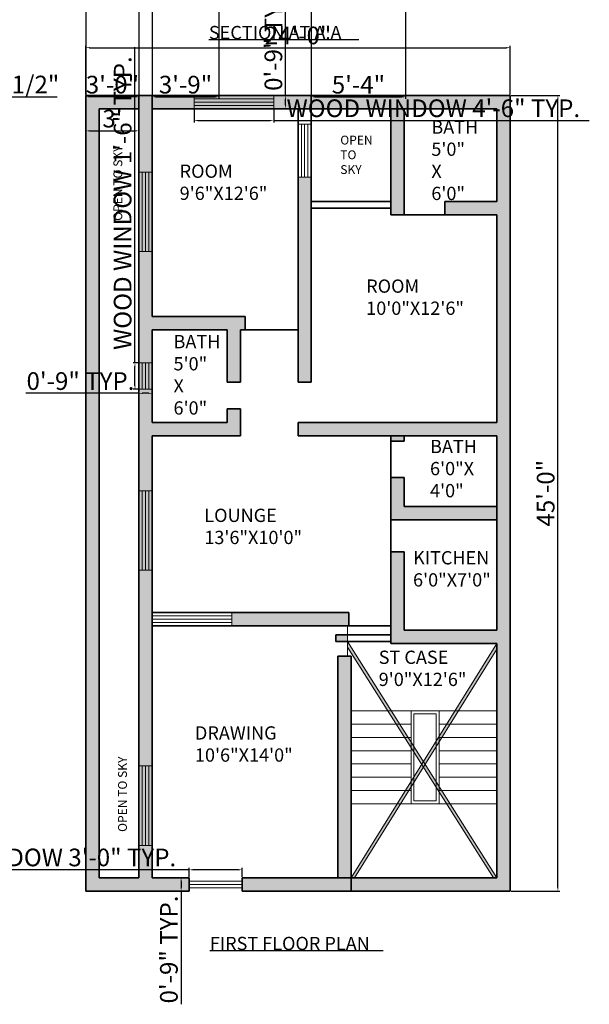
# Model space of a CAD drawing. Units: inches. Extents: x 2693 to 3501, y 1190 to 2292.
# Tile 2 of 4: x 3068 to 3455, y 1190 to 1858. Entities that reach past the tile are written whole.
import ezdxf

# ---------------------------------------------------------------- set-up
doc = ezdxf.new("R2010")
doc.units = ezdxf.units.IN
for name, color, linetype, lineweight in [('A-ANNO-DIMS', 2, 'Continuous', 18), ('A-ANNO-TEXT', 7, 'Continuous', 25), ('A-AREA-IDEN', 7, 'Continuous', 18), ('A-FLOR-STRS', 7, 'Continuous', 18), ('A-FLOR-STRS-PATT', 252, 'Continuous', 13), ('A-GLAZ', 4, 'Continuous', 18), ('A-WALL', 7, 'Continuous', 35), ('A-WALL-PATT', 252, 'Continuous', 13)]:
    doc.layers.add(name, color=color, linetype=linetype, lineweight=lineweight)
doc.styles.get("Standard").update_dxf_attribs({"font": 'arial.ttf'})
doc.dimstyles.new('ISO-25', dxfattribs={"dimtxt": 12, "dimasz": 2.5, "dimexe": 1.25, "dimexo": 0.625, "dimtad": 1, "dimdec": 1, "dimlunit": 3, "dimtxsty": 'Standard', "dimcen": 2.5, "dimadec": 0, "dimazin": 0, "dimtfac": 1, "dimtdec": 1, "dimtmove": 0, "dimatfit": 3, "dimfxl": 1, "dimarcsym": 0})

# ---------------------------------------------------------------- blocks, each defined once
blk = doc.blocks.new('Window - Wood Frame 36 in. Wide plan')
for p, q in [((0, 6), (0, 0)), ((0, 4.5), (36, 4.5)), ((36, 6), (36, 0)), ((0, 3), (36, 3)), ((0, 1.5), (36, 1.5))]:
    blk.add_line(p, q)
blk = doc.blocks.new('*D5')
at = {"layer": 'A-ANNO-DIMS', "color": 0, "lineweight": -2, "transparency": 16777216}
for p, q in [((3113.27, 1805.91), (3113.27, 1781.23)), ((3149.27, 1796.91), (3149.27, 1781.23)), ((3115.77, 1782.48), (3146.77, 1782.48))]:
    blk.add_line(p, q, dxfattribs=at)
at = {"layer": 'A-ANNO-DIMS', "color": 0, "transparency": 16777216}
for points in [[(3115.77, 1782.9), (3115.77, 1782.06), (3113.27, 1782.48)], [(3146.77, 1782.9), (3146.77, 1782.06), (3149.27, 1782.48)]]:
    blk.add_solid(points, dxfattribs=at)
at = {"layer": 'Defpoints', "color": 0, "transparency": 16777216}
for p in [(3113.27, 1806.53), (3149.27, 1797.53), (3149.27, 1782.48)]:
    blk.add_point(p, dxfattribs=at)
at = {"layer": 'A-ANNO-DIMS', "color": 0, "transparency": 16777216, "insert": (3131.27, 1789.23), "char_height": 12, "attachment_point": 5}
blk.add_mtext("3'", dxfattribs=at)
blk = doc.blocks.new('*D9')
at = {"layer": 'A-ANNO-DIMS', "color": 0, "lineweight": -2, "transparency": 16777216}
for p, q in [((3186.75, 1796.91), (3186.75, 1788.18)), ((3240.75, 1796.91), (3240.75, 1788.18)), ((3189.25, 1789.43), (3238.25, 1789.43)), ((3240.75, 1789.43), (3455.01, 1789.43))]:
    blk.add_line(p, q, dxfattribs=at)
at = {"layer": 'A-ANNO-DIMS', "color": 0, "transparency": 16777216}
for points in [[(3189.25, 1789.85), (3189.25, 1789.02), (3186.75, 1789.43)], [(3238.25, 1789.85), (3238.25, 1789.02), (3240.75, 1789.43)]]:
    blk.add_solid(points, dxfattribs=at)
at = {"layer": 'Defpoints', "color": 0, "transparency": 16777216}
for p in [(3186.75, 1797.53), (3240.75, 1797.53), (3240.75, 1789.43)]:
    blk.add_point(p, dxfattribs=at)
at = {"layer": 'A-ANNO-DIMS', "color": 0, "transparency": 16777216, "insert": (3349.13, 1796.27), "char_height": 12, "attachment_point": 5}
blk.add_mtext('WOOD WINDOW 4\'-6" TYP.', dxfattribs=at)
blk = doc.blocks.new('*D10')
at = {"layer": 'A-ANNO-DIMS', "color": 0, "lineweight": -2, "transparency": 16777216}
for p, q in [((3248.85, 1806.53), (3248.85, 1883.43)), ((3241.37, 1806.53), (3250.1, 1806.53)), ((3248.85, 1800.03), (3248.85, 1804.03)), ((3241.37, 1797.53), (3250.1, 1797.53))]:
    blk.add_line(p, q, dxfattribs=at)
at = {"layer": 'A-ANNO-DIMS', "color": 0, "transparency": 16777216}
for points in [[(3248.43, 1804.03), (3249.26, 1804.03), (3248.85, 1806.53)], [(3248.43, 1800.03), (3249.26, 1800.03), (3248.85, 1797.53)]]:
    blk.add_solid(points, dxfattribs=at)
at = {"layer": 'Defpoints', "color": 0, "transparency": 16777216}
for p in [(3240.75, 1806.53), (3248.85, 1806.53), (3240.75, 1797.53)]:
    blk.add_point(p, dxfattribs=at)
at = {"layer": 'A-ANNO-DIMS', "color": 0, "transparency": 16777216, "insert": (3242.09, 1846.23), "char_height": 12, "attachment_point": 5, "rotation": 90}
blk.add_mtext('0\'-9" TYP.', dxfattribs=at)
blk = doc.blocks.new('*D11')
at = {"layer": 'A-ANNO-DIMS', "color": 0, "lineweight": -2, "transparency": 16777216}
for p, q in [((3183.29, 1280.93), (2969.02, 1280.93)), ((3183.29, 1276.16), (3183.29, 1282.18)), ((3216.79, 1280.93), (3185.79, 1280.93)), ((3219.29, 1276.16), (3219.29, 1282.18))]:
    blk.add_line(p, q, dxfattribs=at)
at = {"layer": 'A-ANNO-DIMS', "color": 0, "transparency": 16777216}
for points in [[(3185.79, 1281.35), (3185.79, 1280.52), (3183.29, 1280.93)], [(3216.79, 1281.35), (3216.79, 1280.52), (3219.29, 1280.93)]]:
    blk.add_solid(points, dxfattribs=at)
at = {"layer": 'Defpoints', "color": 0, "transparency": 16777216}
for p in [(3183.29, 1280.93), (3183.29, 1275.53), (3219.29, 1275.53)]:
    blk.add_point(p, dxfattribs=at)
at = {"layer": 'A-ANNO-DIMS', "color": 0, "transparency": 16777216, "insert": (3074.91, 1287.77), "char_height": 12, "attachment_point": 5}
blk.add_mtext('WOOD WINDOW 3\'-0" TYP.', dxfattribs=at)
blk = doc.blocks.new('*D12')
at = {"layer": 'A-ANNO-DIMS', "color": 0, "lineweight": -2, "transparency": 16777216}
for p, q in [((3182.66, 1275.53), (3176.64, 1275.53)), ((3177.89, 1273.03), (3177.89, 1269.03)), ((3182.66, 1266.53), (3176.64, 1266.53)), ((3177.89, 1266.53), (3177.89, 1189.64))]:
    blk.add_line(p, q, dxfattribs=at)
at = {"layer": 'A-ANNO-DIMS', "color": 0, "transparency": 16777216}
for points in [[(3177.47, 1273.03), (3178.31, 1273.03), (3177.89, 1275.53)], [(3177.47, 1269.03), (3178.31, 1269.03), (3177.89, 1266.53)]]:
    blk.add_solid(points, dxfattribs=at)
at = {"layer": 'Defpoints', "color": 0, "transparency": 16777216}
for p in [(3183.29, 1275.53), (3177.89, 1266.53), (3183.29, 1266.53)]:
    blk.add_point(p, dxfattribs=at)
at = {"layer": 'A-ANNO-DIMS', "color": 0, "transparency": 16777216, "insert": (3171.14, 1226.84), "char_height": 12, "attachment_point": 5, "rotation": 90}
blk.add_mtext('0\'-9" TYP.', dxfattribs=at)
blk = doc.blocks.new('*D13')
at = {"layer": 'A-ANNO-DIMS', "color": 0, "lineweight": -2, "transparency": 16777216}
for p, q in [((3146.57, 1625.05), (3146.57, 1839.31)), ((3148.65, 1625.05), (3145.32, 1625.05)), ((3146.57, 1609.55), (3146.57, 1622.55)), ((3148.65, 1607.05), (3145.32, 1607.05))]:
    blk.add_line(p, q, dxfattribs=at)
at = {"layer": 'A-ANNO-DIMS', "color": 0, "transparency": 16777216}
for points in [[(3146.16, 1622.55), (3146.99, 1622.55), (3146.57, 1625.05)], [(3146.16, 1609.55), (3146.99, 1609.55), (3146.57, 1607.05)]]:
    blk.add_solid(points, dxfattribs=at)
at = {"layer": 'Defpoints', "color": 0, "transparency": 16777216}
for p in [(3146.57, 1625.05), (3149.27, 1625.05), (3149.27, 1607.05)]:
    blk.add_point(p, dxfattribs=at)
at = {"layer": 'A-ANNO-DIMS', "color": 0, "transparency": 16777216, "insert": (3139.74, 1733.43), "char_height": 12, "attachment_point": 5, "rotation": 90}
blk.add_mtext('WOOD WINDOW 1\'-6" TYP.', dxfattribs=at)
blk = doc.blocks.new('*D14')
at = {"layer": 'A-ANNO-DIMS', "color": 0, "lineweight": -2, "transparency": 16777216}
for p, q in [((3149.27, 1604.35), (3072.38, 1604.35)), ((3149.27, 1606.42), (3149.27, 1603.1)), ((3155.77, 1604.35), (3151.77, 1604.35)), ((3158.27, 1606.42), (3158.27, 1603.1))]:
    blk.add_line(p, q, dxfattribs=at)
at = {"layer": 'A-ANNO-DIMS', "color": 0, "transparency": 16777216}
for points in [[(3151.77, 1604.76), (3151.77, 1603.93), (3149.27, 1604.35)], [(3155.77, 1604.76), (3155.77, 1603.93), (3158.27, 1604.35)]]:
    blk.add_solid(points, dxfattribs=at)
at = {"layer": 'Defpoints', "color": 0, "transparency": 16777216}
for p in [(3149.27, 1607.05), (3149.27, 1604.35), (3158.27, 1607.05)]:
    blk.add_point(p, dxfattribs=at)
at = {"layer": 'A-ANNO-DIMS', "color": 0, "transparency": 16777216, "insert": (3109.57, 1611.1), "char_height": 12, "attachment_point": 5}
blk.add_mtext('0\'-9" TYP.', dxfattribs=at)
blk = doc.blocks.new('*D30')
at = {"layer": 'A-ANNO-DIMS', "color": 0, "lineweight": -2, "transparency": 16777216}
for p, q in [((3113.27, 1807.16), (3113.27, 1840.18)), ((3115.77, 1838.93), (3398.77, 1838.93)), ((3401.27, 1807.16), (3401.27, 1840.18))]:
    blk.add_line(p, q, dxfattribs=at)
at = {"layer": 'A-ANNO-DIMS', "color": 0, "transparency": 16777216}
for points in [[(3115.77, 1839.35), (3115.77, 1838.52), (3113.27, 1838.93)], [(3398.77, 1839.35), (3398.77, 1838.52), (3401.27, 1838.93)]]:
    blk.add_solid(points, dxfattribs=at)
at = {"layer": 'Defpoints', "color": 0, "transparency": 16777216}
for p in [(3401.27, 1838.93), (3113.27, 1806.53), (3401.27, 1806.53)]:
    blk.add_point(p, dxfattribs=at)
at = {"layer": 'A-ANNO-DIMS', "color": 0, "transparency": 16777216, "insert": (3257.27, 1845.69), "char_height": 12, "attachment_point": 5}
blk.add_mtext('24\'-0"', dxfattribs=at)
blk = doc.blocks.new('*D31')
at = {"layer": 'A-ANNO-DIMS', "color": 0, "lineweight": -2, "transparency": 16777216}
for p, q in [((3401.9, 1806.53), (3434.92, 1806.53)), ((3433.67, 1269.03), (3433.67, 1804.03)), ((3401.9, 1266.53), (3434.92, 1266.53))]:
    blk.add_line(p, q, dxfattribs=at)
at = {"layer": 'A-ANNO-DIMS', "color": 0, "transparency": 16777216}
for points in [[(3433.26, 1804.03), (3434.09, 1804.03), (3433.67, 1806.53)], [(3433.26, 1269.03), (3434.09, 1269.03), (3433.67, 1266.53)]]:
    blk.add_solid(points, dxfattribs=at)
at = {"layer": 'Defpoints', "color": 0, "transparency": 16777216}
for p in [(3401.27, 1806.53), (3433.67, 1806.53), (3401.27, 1266.53)]:
    blk.add_point(p, dxfattribs=at)
at = {"layer": 'A-ANNO-DIMS', "color": 0, "transparency": 16777216, "insert": (3426.92, 1536.53), "char_height": 12, "attachment_point": 5, "rotation": 90}
blk.add_mtext('45\'-0"', dxfattribs=at)
blk = doc.blocks.new('*D41')
at = {"layer": 'A-ANNO-DIMS', "color": 0, "lineweight": -2, "transparency": 16777216}
for p, q in [((2978.99, 1889.87), (2978.99, 1804.29)), ((3029.68, 1889.87), (3029.68, 1804.29)), ((2981.49, 1805.54), (3027.18, 1805.54)), ((3029.68, 1805.54), (3093.77, 1805.54))]:
    blk.add_line(p, q, dxfattribs=at)
at = {"layer": 'A-ANNO-DIMS', "color": 0, "transparency": 16777216}
for points in [[(2981.49, 1805.95), (2981.49, 1805.12), (2978.99, 1805.54)], [(3027.18, 1805.95), (3027.18, 1805.12), (3029.68, 1805.54)]]:
    blk.add_solid(points, dxfattribs=at)
at = {"layer": 'Defpoints', "color": 0, "transparency": 16777216}
for p in [(2978.99, 1890.49), (3029.68, 1890.49), (3029.68, 1805.54)]:
    blk.add_point(p, dxfattribs=at)
at = {"layer": 'A-ANNO-DIMS', "color": 0, "transparency": 16777216, "insert": (3062.97, 1812.37), "char_height": 12, "attachment_point": 5}
blk.add_mtext('4\'-2 1/2"', dxfattribs=at)
blk = doc.blocks.new('*D52')
at = {"layer": 'A-ANNO-DIMS', "color": 0, "lineweight": -2, "transparency": 16777216}
for p, q in [((3149.27, 1887.09), (3149.27, 1804.29)), ((3113.27, 1863.09), (3113.27, 1804.29)), ((3146.77, 1805.54), (3115.77, 1805.54))]:
    blk.add_line(p, q, dxfattribs=at)
at = {"layer": 'A-ANNO-DIMS', "color": 0, "transparency": 16777216}
for points in [[(3115.77, 1805.95), (3115.77, 1805.12), (3113.27, 1805.54)], [(3146.77, 1805.95), (3146.77, 1805.12), (3149.27, 1805.54)]]:
    blk.add_solid(points, dxfattribs=at)
at = {"layer": 'Defpoints', "color": 0, "transparency": 16777216}
for p in [(3149.27, 1887.72), (3113.27, 1863.72), (3113.27, 1805.54)]:
    blk.add_point(p, dxfattribs=at)
at = {"layer": 'A-ANNO-DIMS', "color": 0, "transparency": 16777216, "insert": (3131.27, 1812.29), "char_height": 12, "attachment_point": 5}
blk.add_mtext('3\'-0"', dxfattribs=at)
blk = doc.blocks.new('*D54')
at = {"layer": 'A-ANNO-DIMS', "color": 0, "lineweight": -2, "transparency": 16777216}
for p, q in [((3203.45, 1937.47), (3203.45, 1804.29)), ((3158.27, 1887.09), (3158.27, 1804.29)), ((3160.77, 1805.54), (3200.95, 1805.54))]:
    blk.add_line(p, q, dxfattribs=at)
at = {"layer": 'A-ANNO-DIMS', "color": 0, "transparency": 16777216}
for points in [[(3160.77, 1805.95), (3160.77, 1805.12), (3158.27, 1805.54)], [(3200.95, 1805.95), (3200.95, 1805.12), (3203.45, 1805.54)]]:
    blk.add_solid(points, dxfattribs=at)
at = {"layer": 'Defpoints', "color": 0, "transparency": 16777216}
for p in [(3203.45, 1938.1), (3158.27, 1887.72), (3203.45, 1805.54)]:
    blk.add_point(p, dxfattribs=at)
at = {"layer": 'A-ANNO-DIMS', "color": 0, "transparency": 16777216, "insert": (3180.86, 1812.29), "char_height": 12, "attachment_point": 5}
blk.add_mtext('3\'-9"', dxfattribs=at)
blk = doc.blocks.new('*D55')
at = {"layer": 'A-ANNO-DIMS', "color": 0, "lineweight": -2, "transparency": 16777216}
for p, q in [((3266.27, 1887.09), (3266.27, 1804.29)), ((3330.27, 1887.09), (3330.27, 1804.29)), ((3268.77, 1805.54), (3327.77, 1805.54))]:
    blk.add_line(p, q, dxfattribs=at)
at = {"layer": 'A-ANNO-DIMS', "color": 0, "transparency": 16777216}
for points in [[(3268.77, 1805.95), (3268.77, 1805.12), (3266.27, 1805.54)], [(3327.77, 1805.95), (3327.77, 1805.12), (3330.27, 1805.54)]]:
    blk.add_solid(points, dxfattribs=at)
at = {"layer": 'Defpoints', "color": 0, "transparency": 16777216}
for p in [(3266.27, 1887.72), (3330.27, 1887.72), (3330.27, 1805.54)]:
    blk.add_point(p, dxfattribs=at)
at = {"layer": 'A-ANNO-DIMS', "color": 0, "transparency": 16777216, "insert": (3298.27, 1812.26), "char_height": 12, "attachment_point": 5}
blk.add_mtext('5\'-4"', dxfattribs=at)

msp = doc.modelspace()

# ---------------------------------------------------------------- hatches: boundary and pattern name
at = {"layer": 'A-FLOR-STRS-PATT'}
h = msp.add_hatch(color=256, dxfattribs=at)
h.dxf.hatch_style = 1
h.paths.add_polyline_path([(3290.81, 1435.82), (3290.81, 1432.08), (3318.21, 1388.79), (3320.58, 1388.79)])
h.paths.add_polyline_path([(3392.27, 1430.75), (3392.27, 1434.53), (3363.79, 1388.79), (3366.14, 1388.79)])
h.paths.add_polyline_path([(3366.14, 1388.79), (3363.79, 1388.79), (3358.18, 1379.79), (3360.54, 1379.79)])
h.paths.add_polyline_path([(3360.54, 1379.79), (3358.18, 1379.79), (3353.03, 1371.5), (3353.03, 1370.79), (3354.94, 1370.79)])
h.paths.add_polyline_path([(3351.03, 1364.51), (3351.03, 1368.29), (3342.36, 1354.38), (3343.55, 1352.5)])
h.paths.add_polyline_path([(3353.03, 1371.5), (3351.03, 1368.29), (3351.03, 1364.51), (3353.03, 1367.72)])
h.paths.add_polyline_path([(3354.94, 1370.79), (3353.03, 1370.79), (3353.03, 1367.72)])
h.paths.add_polyline_path([(3326.92, 1325.79), (3324.56, 1325.79), (3293.27, 1275.53), (3295.63, 1275.53)])
h.paths.add_polyline_path([(3332.52, 1334.79), (3330.17, 1334.79), (3324.56, 1325.79), (3326.92, 1325.79)])
h.paths.add_polyline_path([(3333.97, 1337.11), (3333.97, 1340.89), (3330.17, 1334.79), (3332.52, 1334.79)])
h.paths.add_polyline_path([(3335.97, 1344.11), (3333.97, 1340.89), (3333.97, 1337.11), (3335.97, 1340.32)])
h.paths.add_polyline_path([(3342.38, 1350.62), (3341.19, 1352.49), (3335.97, 1344.11), (3335.97, 1340.32)])
h.paths.add_polyline_path([(3335.97, 1364.48), (3335.97, 1360.74), (3341.19, 1352.49), (3342.36, 1354.38)])
h.paths.add_polyline_path([(3343.55, 1352.5), (3342.36, 1354.38), (3341.19, 1352.49), (3342.38, 1350.62)])
h.paths.add_polyline_path([(3343.55, 1352.5), (3342.38, 1350.62), (3351.03, 1336.96), (3351.03, 1340.7)])
h.paths.add_polyline_path([(3331.98, 1370.79), (3329.61, 1370.79), (3333.97, 1363.9), (3333.97, 1367.64)])
h.paths.add_polyline_path([(3333.97, 1367.64), (3333.97, 1363.9), (3335.97, 1360.74), (3335.97, 1364.48)])
h.paths.add_polyline_path([(3326.28, 1379.79), (3323.91, 1379.79), (3329.61, 1370.79), (3331.98, 1370.79)])
h.paths.add_polyline_path([(3353.03, 1337.54), (3351.03, 1340.7), (3351.03, 1336.96), (3353.03, 1333.8)])
h.paths.add_polyline_path([(3353.03, 1337.54), (3353.03, 1334.79), (3354.76, 1334.79)])
h.paths.add_polyline_path([(3354.76, 1334.79), (3353.03, 1334.79), (3353.03, 1333.8), (3358.09, 1325.79), (3360.46, 1325.79)])
h.paths.add_polyline_path([(3360.46, 1325.79), (3358.09, 1325.79), (3389.91, 1275.53), (3392.27, 1275.53)])
h.paths.add_polyline_path([(3320.58, 1388.79), (3318.21, 1388.79), (3323.91, 1379.79), (3326.28, 1379.79)])
at = {"layer": 'A-WALL-PATT'}
h = msp.add_hatch(color=256, dxfattribs=at)
h.dxf.hatch_style = 1
h.paths.add_polyline_path([(3158.27, 1575.53), (3218.27, 1575.53), (3218.27, 1593.71), (3209.27, 1593.71), (3209.27, 1584.53), (3158.27, 1584.53), (3158.27, 1647.53), (3209.27, 1647.53), (3209.27, 1612.01), (3218.27, 1612.01), (3218.27, 1647.53), (3221.27, 1647.53), (3221.27, 1656.53), (3158.27, 1656.53), (3158.27, 1797.53), (3392.27, 1797.53), (3392.27, 1734.53), (3356.93, 1734.53), (3356.93, 1725.53), (3392.27, 1725.53), (3392.27, 1584.53), (3257.27, 1584.53), (3257.27, 1575.53), (3392.27, 1575.53), (3392.27, 1443.53), (3329.27, 1443.53), (3329.27, 1496.68), (3320.27, 1496.68), (3320.27, 1434.53), (3392.27, 1434.53), (3392.27, 1275.53), (3293.27, 1275.53), (3293.27, 1266.53), (3401.27, 1266.53), (3401.27, 1806.53), (3113.27, 1806.53), (3113.27, 1266.53), (3183.29, 1266.53), (3183.29, 1275.53), (3158.27, 1275.53)])
h.paths.add_polyline_path([(3122.27, 1797.53), (3149.27, 1797.53), (3149.27, 1275.53), (3122.27, 1275.53)], flags=16)
h.paths.add_polyline_path([(3158.27, 1484.23), (3149.27, 1484.23), (3149.27, 1351.51), (3158.27, 1351.51)], flags=17)
h.paths.add_polyline_path([(3291.67, 1455.53), (3212.27, 1455.53), (3212.27, 1446.53), (3291.67, 1446.53)], flags=17)
h.paths.add_polyline_path([(3293.27, 1275.53), (3219.29, 1275.53), (3219.29, 1266.53), (3293.27, 1266.53)], flags=17)
h.paths.add_polyline_path([(3266.27, 1725.53), (3266.27, 1751.01), (3257.27, 1751.01), (3257.27, 1647.53), (3257.27, 1612.01), (3266.27, 1612.01)], flags=17)
h.paths.add_polyline_path([(3329.27, 1797.53), (3320.27, 1797.53), (3320.27, 1725.53), (3329.27, 1725.53)], flags=17)
h.paths.add_polyline_path([(3144.47, 1304.74), (3144.47, 1364.57), (3132.11, 1364.57), (3132.11, 1304.74)], flags=8)
h.paths.add_polyline_path([(3141.32, 1719.54), (3141.32, 1779.36), (3128.95, 1779.36), (3128.95, 1719.54)], flags=8)
h = msp.add_hatch(color=256, dxfattribs=at)
h.dxf.hatch_style = 1
h.paths.add_polyline_path([(3329.27, 1575.53), (3320.27, 1575.53), (3320.27, 1571.93), (3329.27, 1571.93)])
h.paths.add_polyline_path([(3329.27, 1547.28), (3320.27, 1547.28), (3320.27, 1518.53), (3392.27, 1518.53), (3392.27, 1527.53), (3329.27, 1527.53)])
h = msp.add_hatch(color=256, dxfattribs=at)
h.dxf.hatch_style = 1
h.paths.add_polyline_path([(3158.27, 1484.23), (3149.27, 1484.23), (3149.27, 1351.51), (3158.27, 1351.51)])
h = msp.add_hatch(color=256, dxfattribs=at)
h.dxf.hatch_style = 1
h.paths.add_polyline_path([(3293.27, 1426.01), (3284.27, 1426.01), (3284.27, 1275.53), (3293.27, 1275.53)])
h.paths.add_polyline_path([(3290.81, 1440.32), (3282.91, 1440.32), (3282.91, 1435.82), (3290.81, 1435.82)])
h.paths.add_polyline_path([(2941.25, 1422.49), (2932.25, 1422.49), (2932.25, 1272.02), (2941.25, 1272.02)])
h.paths.add_polyline_path([(2938.79, 1436.8), (2930.89, 1436.8), (2930.89, 1432.3), (2938.79, 1432.3)])

# ---------------------------------------------------------------- linework, layer by layer
at = {"layer": 'A-ANNO-TEXT'}
for p, q in [((3196.75, 1844.38), (3298.61, 1844.38)), ((3197.38, 1226.11), (3313.12, 1226.11)), ((3313.12, 1226.11), (3315.01, 1226.11))]:
    msp.add_line(p, q, dxfattribs=at)
at = {"layer": 'A-FLOR-STRS'}
for p, q in [((3290.81, 1446.53), (3290.81, 1426.01)), ((3290.81, 1435.82), (3392.27, 1275.53)), ((3290.81, 1432.08), (3389.91, 1275.53)), ((3392.27, 1434.53), (3293.27, 1275.53)), ((3392.27, 1430.75), (3295.63, 1275.53)), ((3293.27, 1388.79), (3392.27, 1388.79)), ((3293.27, 1379.79), (3333.97, 1379.79)), ((3353.03, 1379.79), (3392.27, 1379.79)), ((3293.27, 1370.79), (3333.97, 1370.79)), ((3353.03, 1370.79), (3392.27, 1370.79)), ((3293.27, 1361.79), (3333.97, 1361.79)), ((3353.03, 1361.79), (3392.27, 1361.79)), ((3293.27, 1352.79), (3333.97, 1352.79)), ((3353.03, 1352.79), (3392.27, 1352.79)), ((3293.27, 1343.79), (3333.97, 1343.79)), ((3353.03, 1343.79), (3392.27, 1343.79)), ((3293.27, 1334.79), (3333.97, 1334.79)), ((3353.03, 1334.79), (3392.27, 1334.79)), ((3293.27, 1325.79), (3392.27, 1325.79))]:
    msp.add_line(p, q, dxfattribs=at)
for points in [[(3333.97, 1388.79), (3353.03, 1388.79), (3353.03, 1325.79), (3333.97, 1325.79)], [(3335.97, 1386.79), (3351.03, 1386.79), (3351.03, 1327.79), (3335.97, 1327.79)]]:
    msp.add_lwpolyline(points, close=True, dxfattribs=at)
at = {"layer": 'A-WALL'}
for p, q in [((3113.27, 1806.53), (3401.27, 1806.53)), ((3113.27, 1266.53), (3113.27, 1806.53)), ((3149.27, 1797.53), (3149.27, 1806.53)), ((3158.27, 1797.53), (3158.27, 1806.53)), ((3266.27, 1797.53), (3266.27, 1806.53)), ((3401.27, 1806.53), (3401.27, 1266.53)), ((3122.27, 1275.53), (3122.27, 1797.53)), ((3122.27, 1797.53), (3149.27, 1797.53)), ((3149.27, 1275.53), (3149.27, 1797.53)), ((3158.27, 1656.53), (3158.27, 1797.53)), ((3158.27, 1797.53), (3392.27, 1797.53)), ((3257.27, 1647.53), (3257.27, 1797.53)), ((3266.27, 1725.53), (3266.27, 1797.53)), ((3320.27, 1725.53), (3320.27, 1797.53)), ((3329.27, 1725.53), (3329.27, 1797.53)), ((3392.27, 1797.53), (3392.27, 1734.53)), ((3266.27, 1734.53), (3320.27, 1734.53)), ((3356.93, 1734.53), (3356.93, 1725.53)), ((3356.93, 1734.53), (3392.27, 1734.53)), ((3266.27, 1730.03), (3320.27, 1730.03)), ((3266.27, 1612.01), (3266.27, 1725.53)), ((3320.27, 1725.53), (3392.27, 1725.53)), ((3392.27, 1725.53), (3392.27, 1584.53)), ((3158.27, 1656.53), (3221.27, 1656.53)), ((3221.27, 1647.53), (3221.27, 1656.53)), ((3158.27, 1647.53), (3209.27, 1647.53)), ((3158.27, 1584.53), (3158.27, 1647.53)), ((3209.27, 1612.01), (3209.27, 1647.53)), ((3218.27, 1612.01), (3218.27, 1647.53)), ((3218.27, 1647.53), (3221.27, 1647.53)), ((3218.27, 1647.53), (3257.27, 1647.53)), ((3257.27, 1612.01), (3257.27, 1647.53)), ((3209.27, 1612.01), (3218.27, 1612.01)), ((3257.27, 1612.01), (3266.27, 1612.01)), ((3209.27, 1584.53), (3209.27, 1593.71)), ((3218.27, 1593.71), (3209.27, 1593.71)), ((3218.27, 1575.53), (3218.27, 1593.71)), ((3158.27, 1584.53), (3209.27, 1584.53)), ((3257.27, 1575.53), (3257.27, 1584.53)), ((3257.27, 1584.53), (3392.27, 1584.53)), ((3158.27, 1275.53), (3158.27, 1575.53)), ((3158.27, 1575.53), (3218.27, 1575.53)), ((3257.27, 1575.53), (3392.27, 1575.53)), ((3320.27, 1575.53), (3320.27, 1571.93)), ((3320.27, 1571.93), (3329.27, 1571.93)), ((3320.27, 1547.28), (3320.27, 1571.93)), ((3329.27, 1575.53), (3329.27, 1571.93)), ((3392.27, 1575.53), (3392.27, 1443.53)), ((3320.27, 1547.28), (3329.27, 1547.28)), ((3320.27, 1547.28), (3320.27, 1434.53)), ((3329.27, 1547.28), (3329.27, 1527.53)), ((3329.27, 1527.53), (3392.27, 1527.53)), ((3320.27, 1518.53), (3392.27, 1518.53)), ((3320.27, 1496.68), (3329.27, 1496.68)), ((3329.27, 1496.68), (3329.27, 1443.53)), ((3158.27, 1455.53), (3291.67, 1455.53)), ((3291.67, 1455.53), (3291.67, 1446.53)), ((3158.27, 1446.53), (3320.27, 1446.53)), ((3329.27, 1443.53), (3392.27, 1443.53)), ((3293.27, 1440.32), (3282.91, 1440.32)), ((3284.15, 1440.32), (3282.91, 1440.32)), ((3282.91, 1440.32), (3282.91, 1435.82)), ((3320.13, 1440.32), (3293.27, 1440.32)), ((3282.91, 1435.82), (3293.27, 1435.82)), ((3320.13, 1435.82), (3293.27, 1435.82)), ((3320.27, 1434.53), (3392.27, 1434.53)), ((3392.27, 1434.53), (3392.27, 1275.53)), ((3392.27, 1275.53), (3392.27, 1434.53)), ((3284.27, 1426.01), (3284.27, 1275.53)), ((3284.27, 1426.01), (3293.27, 1426.01)), ((3293.27, 1426.01), (3293.27, 1266.53)), ((3149.27, 1275.53), (3122.27, 1275.53)), ((3183.29, 1275.53), (3158.27, 1275.53)), ((3183.29, 1275.53), (3183.29, 1266.53)), ((3392.27, 1275.53), (3219.29, 1275.53)), ((3219.29, 1266.53), (3219.29, 1275.53)), ((3183.29, 1266.53), (3113.27, 1266.53)), ((3401.27, 1266.53), (3219.29, 1266.53))]:
    msp.add_line(p, q, dxfattribs=at)

# ---------------------------------------------------------------- block references
at = {"layer": 'A-GLAZ', "xscale": 1.5, "yscale": 1.5}
for p in [(3186.75, 1797.53), (3158.27, 1446.53)]:
    msp.add_blockref('Window - Wood Frame 36 in. Wide plan', p, dxfattribs=at)
at = {"layer": 'A-GLAZ', "yscale": 1.5}
for p, rotation in [((3266.27, 1751.01), 90), ((3219.29, 1275.53), 180)]:
    msp.add_blockref('Window - Wood Frame 36 in. Wide plan', p, dxfattribs=dict(at, rotation=rotation))
at = {"layer": 'A-GLAZ', "yscale": 1.5, "rotation": 90}
for p, xscale in [((3158.27, 1700.5), 1.5), ((3158.27, 1607.05), 0.5), ((3158.27, 1484.23), 1.5), ((3158.27, 1297.51), 1.5)]:
    msp.add_blockref('Window - Wood Frame 36 in. Wide plan', p, dxfattribs=dict(at, xscale=xscale))

# ---------------------------------------------------------------- texts
at = {"layer": 'A-ANNO-TEXT', "char_height": 9, "attachment_point": 1}
for s, insert in [('SECTION AT A.A', (3196.75, 1853.69)), ('FIRST FLOOR PLAN', (3197.38, 1235.43))]:
    msp.add_mtext_dynamic_manual_height_columns(s, width=140.9736, gutter_width=12.5, heights=[0], dxfattribs=dict(at, insert=insert))
at = {"layer": 'A-AREA-IDEN', "char_height": 9, "attachment_point": 1}
for s, width, insert in [('BATH\\P5\'0"\\PX\\P6\'0"', 1.6077, (3347.77, 1789.52)), ('ROOM\\P9\'6"X12\'6"', 1.6077, (3176.9, 1759.6)), ('ROOM\\P10\'0"X12\'6"', 1.6077, (3303.54, 1681.6)), ('BATH\\P5\'0"\\PX\\P6\'0"', 1.6077, (3172.73, 1643.9)), ('BATH\\P6\'0"X\\P4\'0"', 1.6077, (3346.88, 1572.76)), ('LOUNGE 13\'6"X10\'0"', 77.2555, (3193.64, 1526.01)), ('KITCHEN\\P6\'0"X7\'0"', 1.6077, (3335.35, 1497.22)), ('ST CASE\\P9\'0"X12\'6"', 77.2555, (3312.03, 1429.68)), ('DRAWING 10\'6"X14\'0"', 77.2555, (3187.28, 1378.32))]:
    msp.add_mtext_dynamic_manual_height_columns(s, width=width, gutter_width=12.5, heights=[0], dxfattribs=dict(at, insert=insert))
at = {"layer": 'A-AREA-IDEN', "insert": (3285.94, 1779.21), "char_height": 6, "attachment_point": 1}
msp.add_mtext('OPEN \\PTO \\PSKY', dxfattribs=at)
at = {"layer": 'A-AREA-IDEN', "char_height": 6, "attachment_point": 1, "rotation": 90}
for insert in [(3131.94, 1721.44), (3135.09, 1306.65)]:
    msp.add_mtext_dynamic_manual_height_columns('OPEN TO SKY', width=75.3875, gutter_width=12.5, heights=[0], dxfattribs=dict(at, insert=insert))

# ---------------------------------------------------------------- dimensions: what is measured, and where the dimension line sits
at = {"layer": 'A-ANNO-DIMS'}
for base, p1, p2, override, picture, middle in [((3203.45, 1805.54), (3158.27, 1887.72), (3203.45, 1938.1), {"dimdec": 1, "dimlfac": 1, "dimrnd": 0, "dimzin": 1, "dimdsep": 46, "dimlunit": 4, "dimfrac": 2}, '*D54', (3180.86, 1812.29)), ((3029.68, 1805.54), (2978.99, 1890.49), (3029.68, 1890.49), {"dimdec": 1, "dimlfac": 1, "dimrnd": 0, "dimzin": 1, "dimdsep": 46, "dimlunit": 4, "dimfrac": 2}, '*D41', (3062.97, 1812.37)), ((3113.27, 1805.54), (3149.27, 1887.72), (3113.27, 1863.72), {"dimdec": 1, "dimlfac": 1, "dimrnd": 0, "dimzin": 1, "dimdsep": 46, "dimlunit": 4, "dimfrac": 2}, '*D52', (3131.27, 1812.29)), ((3330.27, 1805.54), (3266.27, 1887.72), (3330.27, 1887.72), {"dimdec": 1, "dimlfac": 1, "dimrnd": 0, "dimzin": 1, "dimdsep": 46, "dimlunit": 4, "dimfrac": 2}, '*D55', (3298.27, 1812.26)), ((3401.27, 1838.93), (3113.27, 1806.53), (3401.27, 1806.53), {"dimdec": 1, "dimlfac": 1, "dimrnd": 0, "dimzin": 1, "dimdsep": 46, "dimlunit": 4, "dimfrac": 2}, '*D30', (3257.27, 1845.69)), ((3149.27, 1782.48), (3113.27, 1806.53), (3149.27, 1797.53), {"dimclrd": 0, "dimclre": 0, "dimclrt": 0}, '*D5', (3131.27, 1789.23))]:
    dim = msp.add_linear_dim(base=base, p1=p1, p2=p2, dimstyle='ISO-25', override=override, dxfattribs=at)
    dim.commit()
    dim.dimension.update_dxf_attribs({"geometry": picture, "text_midpoint": middle})
for base, p1, p2, angle, text, picture, middle in [((3248.85, 1806.53), (3240.75, 1797.53), (3240.75, 1806.53), 90, '<> TYP.', '*D10', (3242.09, 1846.23)), ((3146.57, 1625.05), (3149.27, 1607.05), (3149.27, 1625.05), 90, 'WOOD WINDOW <> TYP.', '*D13', (3139.74, 1733.43)), ((3149.27, 1604.35), (3158.27, 1607.05), (3149.27, 1607.05), 180, '<> TYP.', '*D14', (3109.57, 1611.1)), ((3183.29, 1280.93), (3219.29, 1275.53), (3183.29, 1275.53), 180, 'WOOD WINDOW <> TYP.', '*D11', (3074.91, 1287.77)), ((3177.89, 1266.53), (3183.29, 1275.53), (3183.29, 1266.53), 270, '<> TYP.', '*D12', (3171.14, 1226.84))]:
    dim = msp.add_linear_dim(base=base, p1=p1, p2=p2, angle=angle, text=text, dimstyle='ISO-25', override={"dimdec": 1, "dimlfac": 1, "dimrnd": 0, "dimzin": 1, "dimdsep": 46, "dimlunit": 4, "dimfrac": 2}, dxfattribs=at)
    dim.commit()
    dim.dimension.update_dxf_attribs({"geometry": picture, "text_midpoint": middle})
dim = msp.add_linear_dim(base=(3240.75, 1789.43), p1=(3186.75, 1797.53), p2=(3240.75, 1797.53), text='WOOD WINDOW <> TYP.', dimstyle='ISO-25', override={"dimdec": 1, "dimlfac": 1, "dimrnd": 0, "dimzin": 1, "dimdsep": 46, "dimlunit": 4, "dimfrac": 2}, dxfattribs=at)
dim.commit()
dim.dimension.update_dxf_attribs({"geometry": '*D9', "text_midpoint": (3349.13, 1796.27)})
dim = msp.add_linear_dim(base=(3433.67, 1806.53), p1=(3401.27, 1266.53), p2=(3401.27, 1806.53), angle=90, dimstyle='ISO-25', override={"dimdec": 1, "dimlfac": 1, "dimrnd": 0, "dimzin": 1, "dimdsep": 46, "dimlunit": 4, "dimfrac": 2}, dxfattribs=at)
dim.commit()
dim.dimension.update_dxf_attribs({"geometry": '*D31', "text_midpoint": (3426.92, 1536.53)})

doc.saveas('drawing.dxf')
